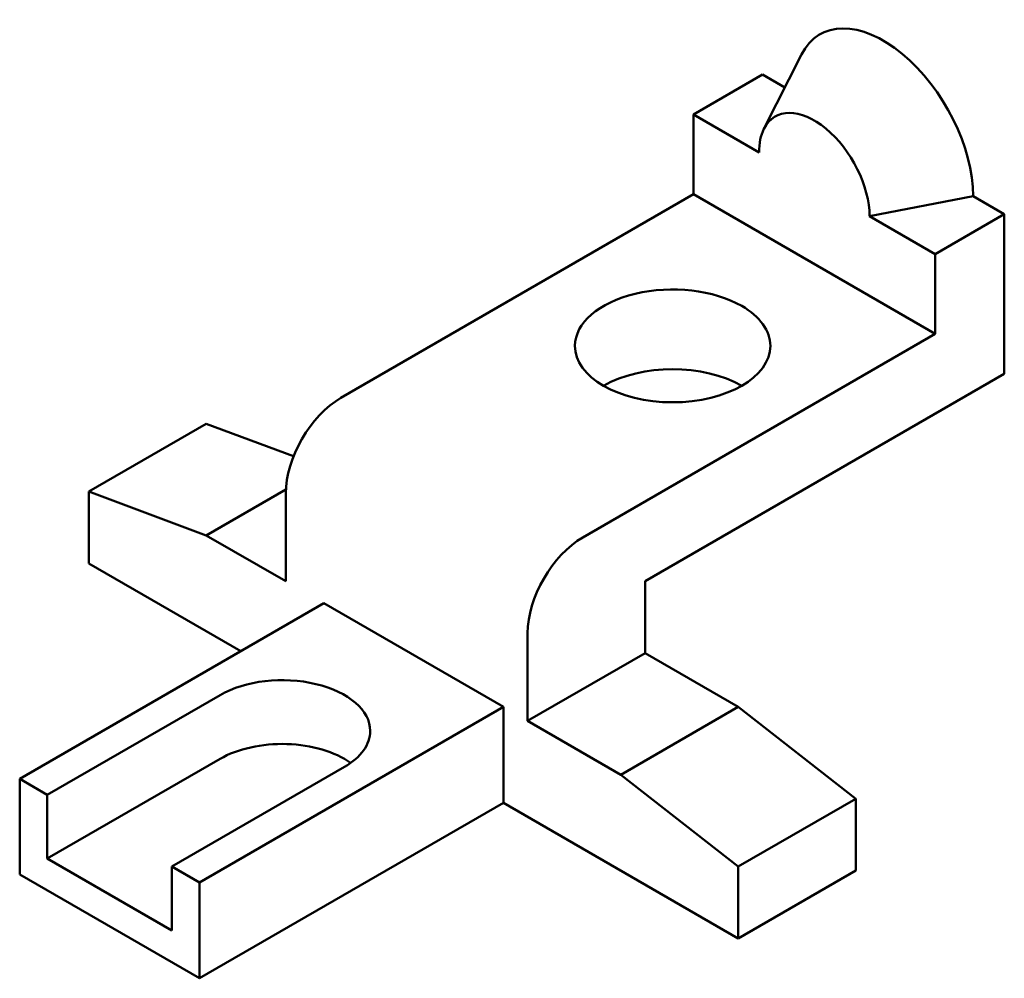
# Model space of a CAD drawing. Units: inches. Extents: x 1177 to 33026, y 779 to 22841.
# Tile 2 of 2: x 29891 to 33026, y 19790 to 22841. Entities that reach past the tile are written whole.
import ezdxf

# ---------------------------------------------------------------- set-up
doc = ezdxf.new("R2010")
doc.units = ezdxf.units.IN
doc.header["$MEASUREMENT"] = 0
doc.layers.add('M-OUTL', color=18, linetype='Continuous', lineweight=50)

msp = doc.modelspace()

# ---------------------------------------------------------------- linework, layer by layer
at = {"layer": 'M-OUTL'}
for p, q in [((32260.2, 22493.8), (32379.9, 22731)), ((32255.6, 22666.9), (32035.6, 22539.9)), ((32326.8, 22625.8), (32255.6, 22666.9)), ((32035.6, 22539.9), (32035.6, 22285.9)), ((32244.6, 22419.2), (32035.6, 22539.9)), ((32035.6, 22285.9), (30913.8, 21638.2)), ((32805.5, 21841.4), (32035.6, 22285.9)), ((32596.6, 22216), (32926.5, 22279.5)), ((33025.5, 22222.4), (32926.5, 22279.5)), ((32805.5, 22095.4), (32596.6, 22216)), ((33025.5, 22222.4), (32805.5, 22095.4)), ((33025.5, 21714.4), (33025.5, 22222.4)), ((32805.5, 22095.4), (32805.5, 21841.4)), ((32805.5, 21841.4), (31683.7, 21193.7)), ((31881.7, 21054), (33025.5, 21714.4)), ((30110.9, 21339.7), (30484.8, 21555.6)), ((30484.8, 21555.6), (30762.7, 21451.8)), ((30110.9, 21339.7), (30484.8, 21200)), ((30110.9, 21111.1), (30110.9, 21339.7)), ((30484.8, 21200), (30738.2, 21346.3)), ((30737.8, 21333.4), (30737.8, 21054)), ((30484.8, 21200), (30737.8, 21054)), ((30594.8, 20831.7), (30110.9, 21111.1)), ((31881.7, 20825.4), (31881.7, 21054)), ((29890.9, 20425.3), (30858.8, 20984.1)), ((31430.7, 20653.9), (30858.8, 20984.1)), ((31507.7, 20888.9), (31507.7, 20609.5)), ((31507.7, 20609.5), (31881.7, 20825.4)), ((31881.7, 20825.4), (32178.6, 20653.9)), ((29978.9, 20374.5), (30528.8, 20692)), ((30462.9, 20095.1), (31430.7, 20653.9)), ((31430.7, 20349.1), (31430.7, 20653.9)), ((31804.7, 20438), (32178.6, 20653.9)), ((32178.6, 20653.9), (32552.6, 20361.8)), ((31507.7, 20609.5), (31804.7, 20438)), ((29978.9, 20171.3), (30528.8, 20488.8)), ((30374.9, 20145.9), (30924.8, 20463.4)), ((31804.7, 20438), (32178.6, 20145.9)), ((29890.9, 20120.5), (29890.9, 20425.3)), ((29978.9, 20374.5), (29890.9, 20425.3)), ((29978.9, 20171.3), (29978.9, 20374.5)), ((30462.9, 19790.3), (31430.7, 20349.1)), ((32178.6, 19917.3), (31430.7, 20349.1)), ((32178.6, 20145.9), (32552.6, 20361.8)), ((32552.6, 20361.8), (32552.6, 20133.2)), ((30374.9, 19942.7), (29978.9, 20171.3)), ((30462.9, 20095.1), (30374.9, 20145.9)), ((30374.9, 19942.7), (30374.9, 20145.9)), ((32178.6, 20145.9), (32178.6, 19917.3)), ((32178.6, 19917.3), (32552.6, 20133.2)), ((30462.9, 19790.3), (29890.9, 20120.5)), ((30462.9, 19790.3), (30462.9, 20095.1))]:
    msp.add_line(p, q, dxfattribs=at)
for centre, major_axis, start_param, end_param in [((32640.6, 22444.6), (202.2, -350.2), 0.785398, 3.50296), ((32420.6, 22317.6), (-124.4, 215.5), 3.926991, 6.644552), ((32420.6, 22317.6), (-124.4, 215.5), 0.361367, 0.785398), ((31969.6, 21803.3), (311.1, 0), 0.785398, 3.141593), ((31969.6, 21803.3), (311.1, 0), 0, 0.785398), ((31969.6, 21803.3), (311.1, 0), 3.141593, 6.283185), ((31969.6, 21549.3), (311.1, 0), 0.785398, 2.356194), ((30913.8, 21435), (124.4, 215.5), 0.785398, 2.356194), ((31683.7, 20990.5), (124.4, 215.5), 0.785398, 2.356194), ((30726.8, 20577.7), (-280, 0), 3.141593, 5.497787), ((30726.8, 20577.7), (-280, 0), 2.356194, 3.141593), ((30726.8, 20374.5), (280, 0), 0.679674, 2.356194)]:
    msp.add_ellipse(centre, major_axis=major_axis, ratio=0.57735, start_param=start_param, end_param=end_param, dxfattribs=at)

doc.saveas('drawing.dxf')
